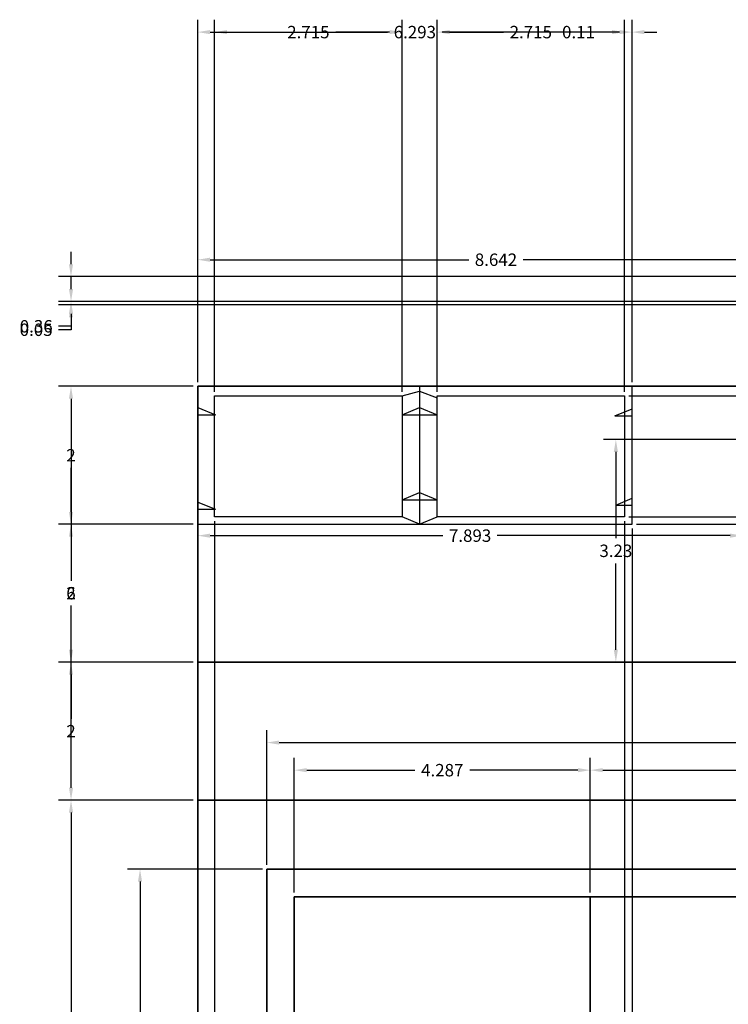
# Model space of a CAD drawing. Units: millimetres. Extents: x 2473 to 2512.3, y 2191.3 to 2230.4.
# Tile 4 of 8: x 2473 to 2483.3, y 2216.1 to 2230.4. Entities that reach past the tile are written whole.
import ezdxf

# ---------------------------------------------------------------- set-up
doc = ezdxf.new("R2010")
doc.units = ezdxf.units.MM
for name, color, linetype, lineweight in [('A-ANNO-DIMS', 2, 'Continuous', 18), ('A-ELEV', 7, 'Continuous', 35), ('A-GLAZ', 3, 'Continuous', 25)]:
    doc.layers.add(name, color=color, linetype=linetype, lineweight=lineweight)
doc.styles.get("Standard").update_dxf_attribs({"font": 'arial.ttf'})
doc.dimstyles.get("Standard").update_dxf_attribs({"dimtxt": 0.18, "dimasz": 0.18, "dimexe": 0.18, "dimexo": 0.0625, "dimgap": 0.09, "dimtad": 0, "dimtih": 1, "dimtoh": 1, "dimdec": 4, "dimzin": 0, "dimdsep": 46, "dimtxsty": 'Standard', "dimcen": 0.09, "dimadec": 0, "dimazin": 0, "dimtfac": 1, "dimtdec": 4, "dimtofl": 0, "dimtmove": 0, "dimatfit": 3, "dimfxl": 1, "dimtolj": 1, "dimtzin": 0, "dimarcsym": 0})

# ---------------------------------------------------------------- blocks, each defined once
blk = doc.blocks.new('*D12')
at = {"layer": 'A-ANNO-DIMS', "color": 0, "lineweight": -2, "transparency": 16777216}
for p, q in [((2475.56, 2219.055), (2473.608, 2219.055)), ((2473.788, 2218.875), (2473.788, 2212.387)), ((2473.788, 2205.535), (2473.788, 2212.023)), ((2475.56, 2205.355), (2473.608, 2205.355))]:
    blk.add_line(p, q, dxfattribs=at)
at = {"layer": 'A-ANNO-DIMS', "color": 0, "transparency": 16777216}
for points in [[(2473.758, 2218.875), (2473.818, 2218.875), (2473.788, 2219.055)], [(2473.758, 2205.535), (2473.818, 2205.535), (2473.788, 2205.355)]]:
    blk.add_solid(points, dxfattribs=at)
at = {"layer": 'Defpoints', "color": 0, "transparency": 16777216}
for p in [(2473.788, 2219.055), (2475.623, 2219.055), (2475.623, 2205.355)]:
    blk.add_point(p, dxfattribs=at)
at = {"layer": 'A-ANNO-DIMS', "color": 0, "transparency": 16777216, "insert": (2473.788, 2212.205), "char_height": 0.18, "attachment_point": 5}
blk.add_mtext('\\A1;13.7', dxfattribs=at)
blk = doc.blocks.new('*D13')
at = {"layer": 'A-ANNO-DIMS', "color": 0, "lineweight": -2, "transparency": 16777216}
for p, q in [((2475.56, 2225.055), (2473.608, 2225.055)), ((2473.788, 2224.875), (2473.788, 2222.237)), ((2473.788, 2219.235), (2473.788, 2221.873)), ((2475.56, 2219.055), (2473.608, 2219.055))]:
    blk.add_line(p, q, dxfattribs=at)
at = {"layer": 'A-ANNO-DIMS', "color": 0, "transparency": 16777216}
for points in [[(2473.758, 2224.875), (2473.818, 2224.875), (2473.788, 2225.055)], [(2473.758, 2219.235), (2473.818, 2219.235), (2473.788, 2219.055)]]:
    blk.add_solid(points, dxfattribs=at)
at = {"layer": 'Defpoints', "color": 0, "transparency": 16777216}
for p in [(2473.788, 2225.055), (2475.623, 2225.055), (2475.623, 2219.055)]:
    blk.add_point(p, dxfattribs=at)
at = {"layer": 'A-ANNO-DIMS', "color": 0, "transparency": 16777216, "insert": (2473.788, 2222.055), "char_height": 0.18, "attachment_point": 5}
blk.add_mtext('\\A1;6', dxfattribs=at)
blk = doc.blocks.new('*D18')
at = {"layer": 'A-ANNO-DIMS', "color": 0, "lineweight": -2, "transparency": 16777216}
for p, q in [((2476.623, 2218.117), (2476.623, 2220.07)), ((2503.664, 2218.117), (2503.664, 2220.07)), ((2476.803, 2219.89), (2489.749, 2219.89)), ((2503.484, 2219.89), (2490.538, 2219.89))]:
    blk.add_line(p, q, dxfattribs=at)
at = {"layer": 'A-ANNO-DIMS', "color": 0, "transparency": 16777216}
for points in [[(2476.803, 2219.92), (2476.803, 2219.86), (2476.623, 2219.89)], [(2503.484, 2219.92), (2503.484, 2219.86), (2503.664, 2219.89)]]:
    blk.add_solid(points, dxfattribs=at)
at = {"layer": 'Defpoints', "color": 0, "transparency": 16777216}
for p in [(2503.664, 2219.89), (2476.623, 2218.055), (2503.664, 2218.055)]:
    blk.add_point(p, dxfattribs=at)
at = {"layer": 'A-ANNO-DIMS', "color": 0, "transparency": 16777216, "insert": (2490.143, 2219.89), "char_height": 0.18, "attachment_point": 5}
blk.add_mtext('\\A1;27.04', dxfattribs=at)
blk = doc.blocks.new('*D19')
at = {"layer": 'A-ANNO-DIMS', "color": 0, "lineweight": -2, "transparency": 16777216}
for p, q in [((2476.56, 2218.055), (2474.608, 2218.055)), ((2474.788, 2217.875), (2474.788, 2212.735)), ((2474.788, 2207.235), (2474.788, 2212.375)), ((2476.56, 2207.055), (2474.608, 2207.055))]:
    blk.add_line(p, q, dxfattribs=at)
at = {"layer": 'A-ANNO-DIMS', "color": 0, "transparency": 16777216}
for points in [[(2474.758, 2217.875), (2474.818, 2217.875), (2474.788, 2218.055)], [(2474.758, 2207.235), (2474.818, 2207.235), (2474.788, 2207.055)]]:
    blk.add_solid(points, dxfattribs=at)
at = {"layer": 'Defpoints', "color": 0, "transparency": 16777216}
for p in [(2474.788, 2218.055), (2476.623, 2218.055), (2476.623, 2207.055)]:
    blk.add_point(p, dxfattribs=at)
at = {"layer": 'A-ANNO-DIMS', "color": 0, "transparency": 16777216, "insert": (2474.788, 2212.555), "char_height": 0.18, "attachment_point": 5}
blk.add_mtext('\\A1;11', dxfattribs=at)
blk = doc.blocks.new('*D21')
at = {"layer": 'A-ANNO-DIMS', "color": 0, "lineweight": -2, "transparency": 16777216}
for p, q in [((2475.623, 2225.117), (2475.623, 2230.37)), ((2481.915, 2225.117), (2481.915, 2230.37)), ((2475.803, 2230.19), (2478.375, 2230.19)), ((2481.735, 2230.19), (2479.163, 2230.19))]:
    blk.add_line(p, q, dxfattribs=at)
at = {"layer": 'A-ANNO-DIMS', "color": 0, "transparency": 16777216}
for points in [[(2475.803, 2230.22), (2475.803, 2230.16), (2475.623, 2230.19)], [(2481.735, 2230.22), (2481.735, 2230.16), (2481.915, 2230.19)]]:
    blk.add_solid(points, dxfattribs=at)
at = {"layer": 'Defpoints', "color": 0, "transparency": 16777216}
for p in [(2481.915, 2230.19), (2475.623, 2225.055), (2481.915, 2225.055)]:
    blk.add_point(p, dxfattribs=at)
at = {"layer": 'A-ANNO-DIMS', "color": 0, "transparency": 16777216, "insert": (2478.769, 2230.19), "char_height": 0.18, "attachment_point": 5}
blk.add_mtext('\\A1;6.293', dxfattribs=at)
blk = doc.blocks.new('*D47')
at = {"layer": 'A-ANNO-DIMS', "color": 0, "lineweight": -2, "transparency": 16777216}
for p, q in [((2477.023, 2217.717), (2477.023, 2219.67)), ((2481.31, 2217.717), (2481.31, 2219.67)), ((2477.203, 2219.49), (2478.769, 2219.49)), ((2481.13, 2219.49), (2479.564, 2219.49))]:
    blk.add_line(p, q, dxfattribs=at)
at = {"layer": 'A-ANNO-DIMS', "color": 0, "transparency": 16777216}
for points in [[(2477.203, 2219.52), (2477.203, 2219.46), (2477.023, 2219.49)], [(2481.13, 2219.52), (2481.13, 2219.46), (2481.31, 2219.49)]]:
    blk.add_solid(points, dxfattribs=at)
at = {"layer": 'Defpoints', "color": 0, "transparency": 16777216}
for p in [(2481.31, 2219.49), (2477.023, 2217.655), (2481.31, 2217.655)]:
    blk.add_point(p, dxfattribs=at)
at = {"layer": 'A-ANNO-DIMS', "color": 0, "transparency": 16777216, "insert": (2479.166, 2219.49), "char_height": 0.18, "attachment_point": 5}
blk.add_mtext('\\A1;4.287', dxfattribs=at)
blk = doc.blocks.new('*D48')
at = {"layer": 'A-ANNO-DIMS', "color": 0, "lineweight": -2, "transparency": 16777216}
for p, q in [((2481.31, 2217.717), (2481.31, 2219.67)), ((2488.479, 2217.717), (2488.479, 2219.67)), ((2481.49, 2219.49), (2484.571, 2219.49)), ((2488.299, 2219.49), (2485.217, 2219.49))]:
    blk.add_line(p, q, dxfattribs=at)
at = {"layer": 'A-ANNO-DIMS', "color": 0, "transparency": 16777216}
for points in [[(2481.49, 2219.52), (2481.49, 2219.46), (2481.31, 2219.49)], [(2488.299, 2219.52), (2488.299, 2219.46), (2488.479, 2219.49)]]:
    blk.add_solid(points, dxfattribs=at)
at = {"layer": 'Defpoints', "color": 0, "transparency": 16777216}
for p in [(2488.479, 2219.49), (2481.31, 2217.655), (2488.479, 2217.655)]:
    blk.add_point(p, dxfattribs=at)
at = {"layer": 'A-ANNO-DIMS', "color": 0, "transparency": 16777216, "insert": (2484.894, 2219.49), "char_height": 0.18, "attachment_point": 5}
blk.add_mtext('\\A1;7.17', dxfattribs=at)
blk = doc.blocks.new('*D68')
at = {"layer": 'A-ANNO-DIMS', "color": 0, "lineweight": -2, "transparency": 16777216}
for p, q in [((2475.56, 2221.055), (2473.608, 2221.055)), ((2473.788, 2220.875), (2473.788, 2220.235)), ((2473.788, 2219.235), (2473.788, 2219.875)), ((2475.56, 2219.055), (2473.608, 2219.055))]:
    blk.add_line(p, q, dxfattribs=at)
at = {"layer": 'A-ANNO-DIMS', "color": 0, "transparency": 16777216}
for points in [[(2473.758, 2220.875), (2473.818, 2220.875), (2473.788, 2221.055)], [(2473.758, 2219.235), (2473.818, 2219.235), (2473.788, 2219.055)]]:
    blk.add_solid(points, dxfattribs=at)
at = {"layer": 'Defpoints', "color": 0, "transparency": 16777216}
for p in [(2473.788, 2221.055), (2475.623, 2221.055), (2475.623, 2219.055)]:
    blk.add_point(p, dxfattribs=at)
at = {"layer": 'A-ANNO-DIMS', "color": 0, "transparency": 16777216, "insert": (2473.788, 2220.055), "char_height": 0.18, "attachment_point": 5}
blk.add_mtext('\\A1;2', dxfattribs=at)
blk = doc.blocks.new('*D69')
at = {"layer": 'A-ANNO-DIMS', "color": 0, "lineweight": -2, "transparency": 16777216}
for p, q in [((2475.56, 2223.055), (2473.608, 2223.055)), ((2473.788, 2222.875), (2473.788, 2222.235)), ((2473.788, 2221.235), (2473.788, 2221.875)), ((2475.56, 2221.055), (2473.608, 2221.055))]:
    blk.add_line(p, q, dxfattribs=at)
at = {"layer": 'A-ANNO-DIMS', "color": 0, "transparency": 16777216}
for points in [[(2473.758, 2222.875), (2473.818, 2222.875), (2473.788, 2223.055)], [(2473.758, 2221.235), (2473.818, 2221.235), (2473.788, 2221.055)]]:
    blk.add_solid(points, dxfattribs=at)
at = {"layer": 'Defpoints', "color": 0, "transparency": 16777216}
for p in [(2473.788, 2223.055), (2475.623, 2223.055), (2475.623, 2221.055)]:
    blk.add_point(p, dxfattribs=at)
at = {"layer": 'A-ANNO-DIMS', "color": 0, "transparency": 16777216, "insert": (2473.788, 2222.055), "char_height": 0.18, "attachment_point": 5}
blk.add_mtext('\\A1;2', dxfattribs=at)
blk = doc.blocks.new('*D70')
at = {"layer": 'A-ANNO-DIMS', "color": 0, "lineweight": -2, "transparency": 16777216}
for p, q in [((2475.56, 2225.055), (2473.608, 2225.055)), ((2473.788, 2224.875), (2473.788, 2224.235)), ((2473.788, 2223.235), (2473.788, 2223.875)), ((2475.56, 2223.055), (2473.608, 2223.055))]:
    blk.add_line(p, q, dxfattribs=at)
at = {"layer": 'A-ANNO-DIMS', "color": 0, "transparency": 16777216}
for points in [[(2473.758, 2224.875), (2473.818, 2224.875), (2473.788, 2225.055)], [(2473.758, 2223.235), (2473.818, 2223.235), (2473.788, 2223.055)]]:
    blk.add_solid(points, dxfattribs=at)
at = {"layer": 'Defpoints', "color": 0, "transparency": 16777216}
for p in [(2473.788, 2225.055), (2475.623, 2225.055), (2475.623, 2223.055)]:
    blk.add_point(p, dxfattribs=at)
at = {"layer": 'A-ANNO-DIMS', "color": 0, "transparency": 16777216, "insert": (2473.788, 2224.055), "char_height": 0.18, "attachment_point": 5}
blk.add_mtext('\\A1;2', dxfattribs=at)
blk = doc.blocks.new('*D71')
at = {"layer": 'A-ANNO-DIMS', "color": 0, "lineweight": -2, "transparency": 16777216}
for p, q in [((2481.806, 2224.977), (2481.806, 2230.37)), ((2481.915, 2225.117), (2481.915, 2230.37)), ((2481.626, 2230.19), (2481.446, 2230.19)), ((2482.095, 2230.19), (2482.275, 2230.19))]:
    blk.add_line(p, q, dxfattribs=at)
at = {"layer": 'A-ANNO-DIMS', "color": 0, "transparency": 16777216}
for points in [[(2481.626, 2230.22), (2481.626, 2230.16), (2481.806, 2230.19)], [(2482.095, 2230.22), (2482.095, 2230.16), (2481.915, 2230.19)]]:
    blk.add_solid(points, dxfattribs=at)
at = {"layer": 'Defpoints', "color": 0, "transparency": 16777216}
for p in [(2481.806, 2230.19), (2481.915, 2225.055), (2481.806, 2224.915)]:
    blk.add_point(p, dxfattribs=at)
at = {"layer": 'A-ANNO-DIMS', "color": 0, "transparency": 16777216, "insert": (2481.14, 2230.19), "char_height": 0.18, "attachment_point": 5}
blk.add_mtext('\\A1;0.11', dxfattribs=at)
blk = doc.blocks.new('*D72')
at = {"layer": 'A-ANNO-DIMS', "color": 0, "lineweight": -2, "transparency": 16777216}
for p, q in [((2475.623, 2225.117), (2475.623, 2227.07)), ((2484.265, 2225.117), (2484.265, 2227.07)), ((2475.803, 2226.89), (2479.551, 2226.89)), ((2484.085, 2226.89), (2480.337, 2226.89))]:
    blk.add_line(p, q, dxfattribs=at)
at = {"layer": 'A-ANNO-DIMS', "color": 0, "transparency": 16777216}
for points in [[(2475.803, 2226.92), (2475.803, 2226.86), (2475.623, 2226.89)], [(2484.085, 2226.92), (2484.085, 2226.86), (2484.265, 2226.89)]]:
    blk.add_solid(points, dxfattribs=at)
at = {"layer": 'Defpoints', "color": 0, "transparency": 16777216}
for p in [(2484.265, 2226.89), (2475.623, 2225.055), (2484.265, 2225.055)]:
    blk.add_point(p, dxfattribs=at)
at = {"layer": 'A-ANNO-DIMS', "color": 0, "transparency": 16777216, "insert": (2479.944, 2226.89), "char_height": 0.18, "attachment_point": 5}
blk.add_mtext('\\A1;8.642', dxfattribs=at)
blk = doc.blocks.new('*D75')
at = {"layer": 'A-ANNO-DIMS', "color": 0, "lineweight": -2, "transparency": 16777216}
for p, q in [((2483.453, 2224.285), (2481.501, 2224.285)), ((2481.681, 2224.105), (2481.681, 2222.852)), ((2481.681, 2221.235), (2481.681, 2222.488)), ((2483.453, 2221.055), (2481.501, 2221.055))]:
    blk.add_line(p, q, dxfattribs=at)
at = {"layer": 'A-ANNO-DIMS', "color": 0, "transparency": 16777216}
for points in [[(2481.651, 2224.105), (2481.711, 2224.105), (2481.681, 2224.285)], [(2481.651, 2221.235), (2481.711, 2221.235), (2481.681, 2221.055)]]:
    blk.add_solid(points, dxfattribs=at)
at = {"layer": 'Defpoints', "color": 0, "transparency": 16777216}
for p in [(2481.681, 2224.285), (2483.516, 2224.285), (2483.516, 2221.055)]:
    blk.add_point(p, dxfattribs=at)
at = {"layer": 'A-ANNO-DIMS', "color": 0, "transparency": 16777216, "insert": (2481.681, 2222.67), "char_height": 0.18, "attachment_point": 5}
blk.add_mtext('\\A1;3.23', dxfattribs=at)
blk = doc.blocks.new('*D77')
at = {"layer": 'A-ANNO-DIMS', "color": 0, "lineweight": -2, "transparency": 16777216}
for p, q in [((2475.623, 2221.117), (2475.623, 2223.07)), ((2483.516, 2221.117), (2483.516, 2223.07)), ((2475.803, 2222.89), (2479.176, 2222.89)), ((2483.336, 2222.89), (2479.962, 2222.89))]:
    blk.add_line(p, q, dxfattribs=at)
at = {"layer": 'A-ANNO-DIMS', "color": 0, "transparency": 16777216}
for points in [[(2475.803, 2222.92), (2475.803, 2222.86), (2475.623, 2222.89)], [(2483.336, 2222.92), (2483.336, 2222.86), (2483.516, 2222.89)]]:
    blk.add_solid(points, dxfattribs=at)
at = {"layer": 'Defpoints', "color": 0, "transparency": 16777216}
for p in [(2483.516, 2222.89), (2475.623, 2221.055), (2483.516, 2221.055)]:
    blk.add_point(p, dxfattribs=at)
at = {"layer": 'A-ANNO-DIMS', "color": 0, "transparency": 16777216, "insert": (2479.569, 2222.89), "char_height": 0.18, "attachment_point": 5}
blk.add_mtext('\\A1;7.893', dxfattribs=at)
blk = doc.blocks.new('*D123')
at = {"layer": 'A-ANNO-DIMS', "color": 0, "lineweight": -2, "transparency": 16777216}
for p, q in [((2473.788, 2226.825), (2473.788, 2227.005)), ((2498.65, 2226.645), (2473.608, 2226.645)), ((2498.79, 2226.285), (2473.608, 2226.285)), ((2473.788, 2226.105), (2473.788, 2225.925)), ((2473.788, 2225.925), (2473.608, 2225.925))]:
    blk.add_line(p, q, dxfattribs=at)
at = {"layer": 'A-ANNO-DIMS', "color": 0, "transparency": 16777216}
for points in [[(2473.758, 2226.825), (2473.818, 2226.825), (2473.788, 2226.645)], [(2473.758, 2226.105), (2473.818, 2226.105), (2473.788, 2226.285)]]:
    blk.add_solid(points, dxfattribs=at)
at = {"layer": 'Defpoints', "color": 0, "transparency": 16777216}
for p in [(2498.713, 2226.645), (2473.788, 2226.285), (2498.852, 2226.285)]:
    blk.add_point(p, dxfattribs=at)
at = {"layer": 'A-ANNO-DIMS', "color": 0, "transparency": 16777216, "insert": (2473.284, 2225.925), "char_height": 0.18, "attachment_point": 5}
blk.add_mtext('\\A1;0.36', dxfattribs=at)
blk = doc.blocks.new('*D124')
at = {"layer": 'A-ANNO-DIMS', "color": 0, "lineweight": -2, "transparency": 16777216}
for p, q in [((2473.788, 2226.465), (2473.788, 2226.645)), ((2498.79, 2226.285), (2473.608, 2226.285)), ((2498.832, 2226.235), (2473.608, 2226.235)), ((2473.788, 2226.055), (2473.788, 2225.875)), ((2473.788, 2225.875), (2473.608, 2225.875))]:
    blk.add_line(p, q, dxfattribs=at)
at = {"layer": 'A-ANNO-DIMS', "color": 0, "transparency": 16777216}
for points in [[(2473.758, 2226.465), (2473.818, 2226.465), (2473.788, 2226.285)], [(2473.758, 2226.055), (2473.818, 2226.055), (2473.788, 2226.235)]]:
    blk.add_solid(points, dxfattribs=at)
at = {"layer": 'Defpoints', "color": 0, "transparency": 16777216}
for p in [(2473.788, 2226.235), (2498.852, 2226.285), (2498.894, 2226.235)]:
    blk.add_point(p, dxfattribs=at)
at = {"layer": 'A-ANNO-DIMS', "color": 0, "transparency": 16777216, "insert": (2473.283, 2225.875), "char_height": 0.18, "attachment_point": 5}
blk.add_mtext('\\A1;0.05', dxfattribs=at)
blk = doc.blocks.new('*D126')
at = {"layer": 'A-ANNO-DIMS', "color": 0, "lineweight": -2, "transparency": 16777216}
for p, q in [((2475.869, 2223.101), (2475.869, 2191.34)), ((2475.623, 2222.992), (2475.623, 2191.34)), ((2475.443, 2191.52), (2475.263, 2191.52)), ((2476.049, 2191.52), (2476.229, 2191.52))]:
    blk.add_line(p, q, dxfattribs=at)
at = {"layer": 'A-ANNO-DIMS', "color": 0, "transparency": 16777216}
for points in [[(2475.443, 2191.55), (2475.443, 2191.49), (2475.623, 2191.52)], [(2476.049, 2191.55), (2476.049, 2191.49), (2475.869, 2191.52)]]:
    blk.add_solid(points, dxfattribs=at)
at = {"layer": 'Defpoints', "color": 0, "transparency": 16777216}
for p in [(2475.623, 2223.055), (2475.869, 2223.163), (2475.869, 2191.52)]:
    blk.add_point(p, dxfattribs=at)
at = {"layer": 'A-ANNO-DIMS', "color": 0, "transparency": 16777216, "insert": (2476.553, 2191.52), "char_height": 0.18, "attachment_point": 5}
blk.add_mtext('\\A1;0.25', dxfattribs=at)
blk = doc.blocks.new('*D127')
at = {"layer": 'A-ANNO-DIMS', "color": 0, "lineweight": -2, "transparency": 16777216}
for p, q in [((2475.869, 2224.977), (2475.869, 2230.37)), ((2478.584, 2224.977), (2478.584, 2230.37)), ((2476.049, 2230.19), (2476.831, 2230.19)), ((2478.404, 2230.19), (2477.622, 2230.19))]:
    blk.add_line(p, q, dxfattribs=at)
at = {"layer": 'A-ANNO-DIMS', "color": 0, "transparency": 16777216}
for points in [[(2476.049, 2230.22), (2476.049, 2230.16), (2475.869, 2230.19)], [(2478.404, 2230.22), (2478.404, 2230.16), (2478.584, 2230.19)]]:
    blk.add_solid(points, dxfattribs=at)
at = {"layer": 'Defpoints', "color": 0, "transparency": 16777216}
for p in [(2478.584, 2230.19), (2475.869, 2224.915), (2478.584, 2224.915)]:
    blk.add_point(p, dxfattribs=at)
at = {"layer": 'A-ANNO-DIMS', "color": 0, "transparency": 16777216, "insert": (2477.226, 2230.19), "char_height": 0.18, "attachment_point": 5}
blk.add_mtext('\\A1;2.715', dxfattribs=at)
blk = doc.blocks.new('*D128')
at = {"layer": 'A-ANNO-DIMS', "color": 0, "lineweight": -2, "transparency": 16777216}
for p, q in [((2479.091, 2224.977), (2479.091, 2230.37)), ((2481.806, 2224.977), (2481.806, 2230.37)), ((2479.271, 2230.19), (2480.053, 2230.19)), ((2481.626, 2230.19), (2480.844, 2230.19))]:
    blk.add_line(p, q, dxfattribs=at)
at = {"layer": 'A-ANNO-DIMS', "color": 0, "transparency": 16777216}
for points in [[(2479.271, 2230.22), (2479.271, 2230.16), (2479.091, 2230.19)], [(2481.626, 2230.22), (2481.626, 2230.16), (2481.806, 2230.19)]]:
    blk.add_solid(points, dxfattribs=at)
at = {"layer": 'Defpoints', "color": 0, "transparency": 16777216}
for p in [(2481.806, 2230.19), (2479.091, 2224.915), (2481.806, 2224.915)]:
    blk.add_point(p, dxfattribs=at)
at = {"layer": 'A-ANNO-DIMS', "color": 0, "transparency": 16777216, "insert": (2480.449, 2230.19), "char_height": 0.18, "attachment_point": 5}
blk.add_mtext('\\A1;2.715', dxfattribs=at)
blk = doc.blocks.new('*D129')
at = {"layer": 'A-ANNO-DIMS', "color": 0, "lineweight": -2, "transparency": 16777216}
for p, q in [((2481.806, 2223.101), (2481.806, 2191.34)), ((2481.915, 2222.992), (2481.915, 2191.34)), ((2481.626, 2191.52), (2481.446, 2191.52)), ((2482.095, 2191.52), (2482.275, 2191.52))]:
    blk.add_line(p, q, dxfattribs=at)
at = {"layer": 'A-ANNO-DIMS', "color": 0, "transparency": 16777216}
for points in [[(2481.626, 2191.55), (2481.626, 2191.49), (2481.806, 2191.52)], [(2482.095, 2191.55), (2482.095, 2191.49), (2481.915, 2191.52)]]:
    blk.add_solid(points, dxfattribs=at)
at = {"layer": 'Defpoints', "color": 0, "transparency": 16777216}
for p in [(2481.806, 2223.163), (2481.915, 2223.055), (2481.915, 2191.52)]:
    blk.add_point(p, dxfattribs=at)
at = {"layer": 'A-ANNO-DIMS', "color": 0, "transparency": 16777216, "insert": (2482.582, 2191.52), "char_height": 0.18, "attachment_point": 5}
blk.add_mtext('\\A1;0.11', dxfattribs=at)
blk = doc.blocks.new('*D130')
at = {"layer": 'A-ANNO-DIMS', "color": 0, "lineweight": -2, "transparency": 16777216}
for p, q in [((2511.548, 2225.235), (2511.548, 2225.415)), ((2481.978, 2225.055), (2511.728, 2225.055)), ((2481.869, 2224.915), (2511.728, 2224.915)), ((2511.548, 2224.735), (2511.548, 2224.555)), ((2511.548, 2224.555), (2511.368, 2224.555))]:
    blk.add_line(p, q, dxfattribs=at)
at = {"layer": 'A-ANNO-DIMS', "color": 0, "transparency": 16777216}
for points in [[(2511.518, 2225.235), (2511.578, 2225.235), (2511.548, 2225.055)], [(2511.518, 2224.735), (2511.578, 2224.735), (2511.548, 2224.915)]]:
    blk.add_solid(points, dxfattribs=at)
at = {"layer": 'Defpoints', "color": 0, "transparency": 16777216}
for p in [(2481.915, 2225.055), (2481.806, 2224.915), (2511.548, 2224.915)]:
    blk.add_point(p, dxfattribs=at)
at = {"layer": 'A-ANNO-DIMS', "color": 0, "transparency": 16777216, "insert": (2511.044, 2224.555), "char_height": 0.18, "attachment_point": 5}
blk.add_mtext('\\A1;0.14', dxfattribs=at)
blk = doc.blocks.new('*D131')
at = {"layer": 'A-ANNO-DIMS', "color": 0, "lineweight": -2, "transparency": 16777216}
for p, q in [((2511.548, 2223.343), (2511.548, 2223.523)), ((2511.548, 2223.523), (2511.728, 2223.523)), ((2481.869, 2223.163), (2511.728, 2223.163)), ((2481.978, 2223.055), (2511.728, 2223.055)), ((2511.548, 2222.875), (2511.548, 2222.695))]:
    blk.add_line(p, q, dxfattribs=at)
at = {"layer": 'A-ANNO-DIMS', "color": 0, "transparency": 16777216}
for points in [[(2511.518, 2223.343), (2511.578, 2223.343), (2511.548, 2223.163)], [(2511.518, 2222.875), (2511.578, 2222.875), (2511.548, 2223.055)]]:
    blk.add_solid(points, dxfattribs=at)
at = {"layer": 'Defpoints', "color": 0, "transparency": 16777216}
for p in [(2481.806, 2223.163), (2481.915, 2223.055), (2511.548, 2223.163)]:
    blk.add_point(p, dxfattribs=at)
at = {"layer": 'A-ANNO-DIMS', "color": 0, "transparency": 16777216, "insert": (2512.034, 2223.523), "char_height": 0.18, "attachment_point": 5}
blk.add_mtext('\\A1;0.11', dxfattribs=at)

msp = doc.modelspace()

# ---------------------------------------------------------------- linework, layer by layer
at = {"layer": 'A-ELEV'}
for p, q in [((2475.6229, 2221.0549), (2475.6229, 2225.0549)), ((2475.6229, 2225.0549), (2484.2649, 2225.0549)), ((2506.7629, 2221.0549), (2475.6229, 2221.0549)), ((2475.6229, 2219.0549), (2475.6229, 2221.0549)), ((2506.7629, 2219.0549), (2475.6229, 2219.0549)), ((2475.6229, 2193.3549), (2475.6229, 2219.0549)), ((2476.6229, 2218.0549), (2476.6229, 2207.0549)), ((2503.6639, 2218.0549), (2476.6229, 2218.0549)), ((2477.0229, 2217.6549), (2477.0229, 2207.4549)), ((2477.0229, 2217.6549), (2503.0616, 2217.6549)), ((2481.3096, 2209.4549), (2481.3096, 2217.6549))]:
    msp.add_line(p, q, dxfattribs=at)
at = {"layer": 'A-GLAZ'}
for p, q in [((2478.834, 2225.0549), (2478.834, 2223.0549)), ((2481.9154, 2223.0549), (2481.9154, 2225.0549)), ((2475.869, 2223.1632), (2475.869, 2224.9147)), ((2475.869, 2224.9147), (2478.584, 2224.9147)), ((2478.584, 2224.9147), (2478.834, 2224.9855)), ((2478.584, 2224.9147), (2478.584, 2223.1632)), ((2478.834, 2224.9855), (2479.0911, 2224.8899)), ((2479.0911, 2223.1632), (2479.0911, 2224.9147)), ((2479.0911, 2224.9147), (2481.806, 2224.9147)), ((2481.806, 2224.9147), (2481.806, 2223.1632)), ((2475.6233, 2224.7486), (2475.8804, 2224.6438)), ((2475.6233, 2224.6438), (2475.8804, 2224.6438)), ((2478.584, 2224.6438), (2478.834, 2224.7486)), ((2478.584, 2224.6438), (2478.834, 2224.6438)), ((2478.834, 2224.7486), (2479.0911, 2224.6438)), ((2478.834, 2224.6438), (2479.0911, 2224.6438)), ((2481.6652, 2224.6253), (2481.9152, 2224.7302)), ((2481.6652, 2224.6253), (2481.9152, 2224.6253)), ((2478.584, 2223.4093), (2478.834, 2223.5142)), ((2478.834, 2223.5142), (2479.0911, 2223.4093)), ((2475.6247, 2223.3775), (2475.8818, 2223.2726)), ((2478.584, 2223.4093), (2478.834, 2223.4093)), ((2478.834, 2223.4093), (2479.0911, 2223.4093)), ((2481.681, 2223.3329), (2481.9154, 2223.4312)), ((2475.6247, 2223.2726), (2475.8818, 2223.2726)), ((2481.681, 2223.3329), (2481.9154, 2223.3329)), ((2475.6229, 2223.0549), (2481.9154, 2223.0549)), ((2478.584, 2223.1632), (2475.869, 2223.1632)), ((2478.834, 2223.0549), (2478.584, 2223.1632)), ((2478.834, 2223.0549), (2479.0911, 2223.1632)), ((2481.806, 2223.1632), (2479.0911, 2223.1632))]:
    msp.add_line(p, q, dxfattribs=at)

# ---------------------------------------------------------------- dimensions: what is measured, and where the dimension line sits
at = {"layer": 'A-ANNO-DIMS'}
for base, p1, p2, override, picture, middle in [((2481.91543, 2230.18989), (2475.6229, 2225.05489), (2481.91543, 2225.05489), {"dimdec": 3, "dimlfac": 1, "dimrnd": 0, "dimzin": 0, "dimdsep": 46, "dimlunit": 2}, '*D21', (2478.76917, 2230.18989)), ((2478.584, 2230.1899), (2475.869, 2224.9147), (2478.584, 2224.9147), {"dimdec": 3, "dimlfac": 1, "dimrnd": 0, "dimzin": 0, "dimdsep": 46, "dimlunit": 2}, '*D127', (2477.2265, 2230.1899)), ((2481.806, 2230.1899), (2479.0911, 2224.9147), (2481.806, 2224.9147), {"dimdec": 3, "dimlfac": 1, "dimrnd": 0, "dimzin": 0, "dimdsep": 46, "dimlunit": 2}, '*D128', (2480.4485, 2230.1899)), ((2481.806, 2230.1899), (2481.9154, 2225.0549), (2481.806, 2224.9147), {"dimdec": 2, "dimlfac": 1, "dimrnd": 0, "dimzin": 0, "dimdsep": 46, "dimlunit": 2}, '*D71', (2481.1396, 2230.1899)), ((2484.2649, 2226.8899), (2475.6229, 2225.0549), (2484.2649, 2225.0549), {"dimdec": 3, "dimlfac": 1, "dimrnd": 0, "dimzin": 0, "dimdsep": 46, "dimlunit": 2}, '*D72', (2479.9439, 2226.8899)), ((2475.869, 2191.5199), (2475.6229, 2223.0549), (2475.869, 2223.1632), {"dimdec": 2, "dimlfac": 1, "dimrnd": 0, "dimzin": 0, "dimdsep": 46, "dimlunit": 2}, '*D126', (2476.5535, 2191.5199)), ((2483.5156, 2222.8899), (2475.6229, 2221.0549), (2483.5156, 2221.0549), {"dimdec": 3, "dimlfac": 1, "dimrnd": 0, "dimzin": 0, "dimdsep": 46, "dimlunit": 2}, '*D77', (2479.5693, 2222.8899)), ((2481.9154, 2191.5199), (2481.806, 2223.1632), (2481.9154, 2223.0549), {"dimdec": 2, "dimlfac": 1, "dimrnd": 0, "dimzin": 0, "dimdsep": 46, "dimlunit": 2}, '*D129', (2482.5818, 2191.5199)), ((2503.6639, 2219.8899), (2476.6229, 2218.0549), (2503.6639, 2218.0549), {"dimdec": 2, "dimlfac": 1, "dimrnd": 0, "dimzin": 0, "dimdsep": 46, "dimlunit": 2}, '*D18', (2490.1434, 2219.8899)), ((2481.3096, 2219.4899), (2477.0229, 2217.6549), (2481.3096, 2217.6549), {"dimdec": 3, "dimlfac": 1, "dimrnd": 0, "dimzin": 0, "dimdsep": 46, "dimlunit": 2}, '*D47', (2479.1663, 2219.4899)), ((2488.4789, 2219.4899), (2481.3096, 2217.6549), (2488.4789, 2217.6549), {"dimdec": 2, "dimlfac": 1, "dimrnd": 0, "dimzin": 0, "dimdsep": 46, "dimlunit": 2}, '*D48', (2484.8943, 2219.4899))]:
    dim = msp.add_linear_dim(base=base, p1=p1, p2=p2, dimstyle='Standard', override=override, dxfattribs=at)
    dim.commit()
    dim.dimension.update_dxf_attribs({"geometry": picture, "text_midpoint": middle})
for base, p1, p2, override, picture, middle in [((2473.7879, 2226.2854), (2498.7129, 2226.6451), (2498.8524, 2226.2854), {"dimdec": 2, "dimlfac": 1, "dimrnd": 0, "dimzin": 0, "dimdsep": 46, "dimlunit": 2}, '*D123', (2473.2842, 2225.9254)), ((2473.7879, 2226.2352), (2498.8524, 2226.2854), (2498.8944, 2226.2352), {"dimdec": 2, "dimlfac": 1, "dimrnd": 0, "dimzin": 0, "dimdsep": 46, "dimlunit": 2}, '*D124', (2473.2834, 2225.8752)), ((2511.5479, 2224.9147), (2481.9154, 2225.0549), (2481.806, 2224.9147), {"dimdec": 2, "dimlfac": 1, "dimrnd": 0, "dimzin": 0, "dimdsep": 46, "dimlunit": 2}, '*D130', (2511.0445, 2224.5547)), ((2473.7879, 2225.0549), (2475.6229, 2219.0549), (2475.6229, 2225.0549), {"dimdec": 0, "dimlfac": 1, "dimrnd": 0, "dimzin": 0, "dimdsep": 46, "dimlunit": 2}, '*D13', (2473.7879, 2222.0549)), ((2473.7879, 2225.0549), (2475.6229, 2223.0549), (2475.6229, 2225.0549), {"dimdec": 0, "dimlfac": 1, "dimrnd": 0, "dimzin": 0, "dimdsep": 46, "dimlunit": 2}, '*D70', (2473.7879, 2224.0549)), ((2481.6806, 2224.285), (2483.5156, 2221.0549), (2483.5156, 2224.285), {"dimdec": 2, "dimlfac": 1, "dimrnd": 0, "dimzin": 0, "dimdsep": 46, "dimlunit": 2}, '*D75', (2481.6806, 2222.6699)), ((2511.5479, 2223.1632), (2481.9154, 2223.0549), (2481.806, 2223.1632), {"dimdec": 2, "dimlfac": 1, "dimrnd": 0, "dimzin": 0, "dimdsep": 46, "dimlunit": 2}, '*D131', (2512.0343, 2223.5232)), ((2473.7879, 2223.0549), (2475.6229, 2221.0549), (2475.6229, 2223.0549), {"dimdec": 0, "dimlfac": 1, "dimrnd": 0, "dimzin": 0, "dimdsep": 46, "dimlunit": 2}, '*D69', (2473.7879, 2222.0549)), ((2473.7879, 2221.0549), (2475.6229, 2219.0549), (2475.6229, 2221.0549), {"dimdec": 0, "dimlfac": 1, "dimrnd": 0, "dimzin": 0, "dimdsep": 46, "dimlunit": 2}, '*D68', (2473.7879, 2220.0549)), ((2473.7879, 2219.0549), (2475.6229, 2205.3549), (2475.6229, 2219.0549), {"dimdec": 1, "dimlfac": 1, "dimrnd": 0, "dimzin": 0, "dimdsep": 46, "dimlunit": 2}, '*D12', (2473.7879, 2212.2049)), ((2474.7879, 2218.0549), (2476.6229, 2207.0549), (2476.6229, 2218.0549), {"dimdec": 0, "dimlfac": 1, "dimrnd": 0, "dimzin": 0, "dimdsep": 46, "dimlunit": 2}, '*D19', (2474.7879, 2212.5549))]:
    dim = msp.add_linear_dim(base=base, p1=p1, p2=p2, angle=90, dimstyle='Standard', override=override, dxfattribs=at)
    dim.commit()
    dim.dimension.update_dxf_attribs({"geometry": picture, "text_midpoint": middle})

doc.saveas('drawing.dxf')
